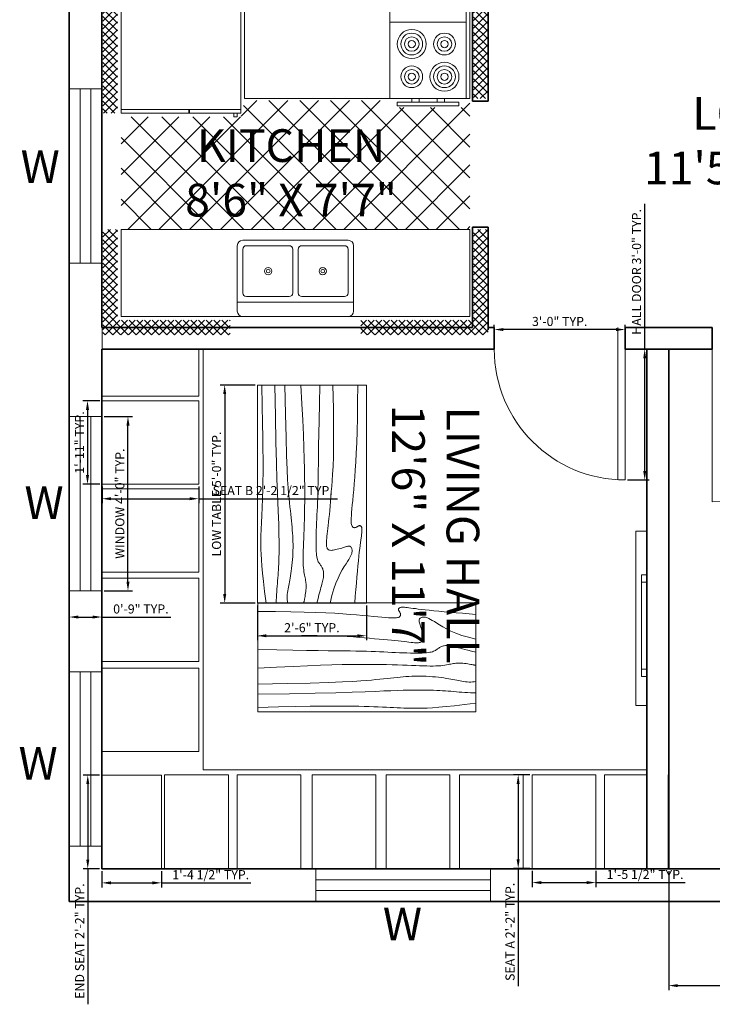
# Model space of a CAD drawing. Units: inches. Extents: x 1642 to 5612, y 1595 to 4064.
# Tile 4 of 6: x 2349 to 2539, y 1708 to 1979. Entities that reach past the tile are written whole.
import ezdxf

# ---------------------------------------------------------------- set-up
doc = ezdxf.new("R2010")
doc.units = ezdxf.units.IN
for name, color, linetype, lineweight in [('A-ANNO-DIMS', 2, 'Continuous', 18), ('A-ANNO-TEXT', 7, 'Continuous', 18), ('A-AREA-IDEN', 7, 'Continuous', 25), ('A-DOOR', 3, 'Continuous', 18), ('A-EQPM', 8, 'Continuous', 13), ('A-FLOR-FIXT', 9, 'Continuous', 18), ('A-FURN', 8, 'Continuous', 13), ('A-GLAZ', 4, 'Continuous', 18), ('A-WALL', 7, 'Continuous', 35)]:
    doc.layers.add(name, color=color, linetype=linetype, lineweight=lineweight)
doc.styles.get("Standard").update_dxf_attribs({"font": 'arial.ttf'})
doc.dimstyles.new('ISO-25', dxfattribs={"dimtxt": 2.5, "dimasz": 2.5, "dimexe": 1.25, "dimexo": 0.625, "dimtad": 1, "dimdec": 0, "dimlunit": 3, "dimtxsty": 'Standard', "dimcen": 2.5, "dimadec": 0, "dimazin": 0, "dimtfac": 1, "dimtdec": 0, "dimtmove": 0, "dimatfit": 3, "dimfxl": 1, "dimarcsym": 0})

# ---------------------------------------------------------------- blocks, each defined once
blk = doc.blocks.new('Kitchen Layout - 7 x 8 ft')
for p, q in [((-5, 81.32), (2.68, 89)), ((-5, 83.44), (0.56, 89)), ((-5, 85.56), (-1.56, 89)), ((-5, 87.68), (-3.68, 89)), ((-1, 84.97), (-5, 88.97)), ((-1, 82.85), (-5, 86.85)), ((1.09, 85), (-2.91, 89)), ((3.21, 85), (-0.79, 89)), ((0.81, 85), (4.81, 89)), ((5.34, 85), (1.34, 89)), ((2.93, 85), (6.93, 89)), ((7.46, 85), (3.46, 89)), ((5.05, 85), (9.05, 89)), ((9.58, 85), (5.58, 89)), ((7.17, 85), (11.17, 89)), ((11.7, 85), (7.7, 89)), ((9.29, 85), (13.29, 89)), ((13.82, 85), (9.82, 89)), ((11.41, 85), (15.41, 89)), ((15.94, 85), (11.94, 89)), ((13.53, 85), (17.53, 89)), ((18.06, 85), (14.06, 89)), ((15.65, 85), (19.65, 89)), ((20.18, 85), (16.18, 89)), ((17.78, 85), (21.78, 89)), ((22.31, 85), (18.31, 89)), ((19.9, 85), (23.9, 89)), ((24.43, 85), (20.43, 89)), ((22.02, 85), (26.02, 89)), ((26.55, 85), (22.55, 89)), ((24.14, 85), (28.14, 89)), ((28.67, 85), (24.67, 89)), ((26.26, 85), (30.26, 89)), ((30.79, 85), (26.79, 89)), ((28.38, 85), (32.38, 89)), ((32.91, 85), (28.91, 89)), ((30.5, 85), (34.5, 89)), ((35.03, 85), (31.03, 89)), ((32.63, 85), (36.63, 89)), ((37.16, 85), (33.16, 89)), ((34.75, 85), (38.75, 89)), ((39.28, 85), (35.28, 89)), ((36.87, 85), (40.87, 89)), ((41.4, 85), (37.4, 89)), ((38.99, 85), (42.99, 89)), ((43.52, 85), (39.52, 89)), ((41.11, 85), (45.11, 89)), ((45.64, 85), (41.64, 89)), ((43.23, 85), (47.23, 89)), ((47.76, 85), (43.76, 89)), ((45.35, 85), (49.35, 89)), ((49.88, 85), (45.88, 89)), ((47.47, 85), (51.47, 89)), ((52, 85), (48, 89)), ((49.6, 85), (53.6, 89)), ((54.13, 85), (50.13, 89)), ((51.72, 85), (55.72, 89)), ((56.25, 85), (52.25, 89)), ((53.84, 85), (57.84, 89)), ((58.37, 85), (54.37, 89)), ((55.96, 85), (59.96, 89)), ((60.49, 85), (56.49, 89)), ((58.08, 85), (62.08, 89)), ((62.61, 85), (58.61, 89)), ((60.2, 85), (64.2, 89)), ((64.73, 85), (60.73, 89)), ((62.32, 85), (66.32, 89)), ((66.85, 85), (62.85, 89)), ((64.45, 85), (68.45, 89)), ((68.97, 85), (64.97, 89)), ((66.57, 85), (70.57, 89)), ((71.1, 85), (67.1, 89)), ((68.69, 85), (72.69, 89)), ((73.22, 85), (69.22, 89)), ((70.81, 85), (74.81, 89)), ((75.34, 85), (71.34, 89)), ((72.93, 85), (76.93, 89)), ((77.46, 85), (73.46, 89)), ((75.05, 85), (79.05, 89)), ((79.58, 85), (75.58, 89)), ((77.17, 85), (81.17, 89)), ((81.7, 85), (77.7, 89)), ((79.29, 85), (83.29, 89)), ((83.82, 85), (79.82, 89)), ((81.42, 85), (85.42, 89)), ((85.95, 85), (81.95, 89)), ((83.54, 85), (87.54, 89)), ((88.07, 85), (84.07, 89)), ((85.66, 85), (89.66, 89)), ((90.19, 85), (86.19, 89)), ((87.78, 85), (91.78, 89)), ((92.31, 85), (88.31, 89)), ((89.9, 85), (93.9, 89)), ((94.43, 85), (90.43, 89)), ((92.02, 85), (96.02, 89)), ((96.55, 85), (92.55, 89)), ((94.14, 85), (98.14, 89)), ((101, 82.67), (94.67, 89)), ((96.27, 85), (100.27, 89)), ((101, 84.79), (96.79, 89)), ((97, 83.61), (101, 87.61)), ((101, 86.92), (98.92, 89)), ((-1, 80.73), (-5, 84.73)), ((34, 84), (96, 84)), ((34, 60), (34, 84)), ((96, 84), (96, 60)), ((97, 81.49), (101, 85.49)), ((101, 80.55), (97, 84.55)), ((-5, 79.19), (-1, 83.19)), ((-1, 78.61), (-5, 82.61)), ((97, 79.37), (101, 83.37)), ((101, 78.43), (97, 82.43)), ((-5, 77.07), (-1, 81.07)), ((-1, 76.49), (-5, 80.49)), ((-5, 74.95), (-1, 78.95)), ((74, 81), (95, 81)), ((97, 77.25), (101, 81.25)), ((101, 76.31), (97, 80.31)), ((97, 75.13), (101, 79.13)), ((-1, 74.36), (-5, 78.36)), ((-5, 72.83), (-1, 76.83)), ((-1, 72.24), (-5, 76.24)), ((101, 74.19), (97, 78.19)), ((97, 73.01), (101, 77.01)), ((101, 72.07), (97, 76.07)), ((-5, 70.71), (-1, 74.71)), ((-1, 70.12), (-5, 74.12)), ((97, 70.89), (101, 74.89)), ((101, 69.95), (97, 73.95)), ((-5, 68.59), (-1, 72.59)), ((-1, 68), (-5, 72)), ((-5, 66.47), (-1, 70.47)), ((97, 68.76), (101, 72.76)), ((101, 67.82), (97, 71.82)), ((97, 66.64), (101, 70.64)), ((-1, 65.88), (-5, 69.88)), ((-5, 64.35), (-1, 68.35)), ((-1, 63.76), (-5, 67.76)), ((101, 65.7), (97, 69.7)), ((97, 64.52), (101, 68.52)), ((-5, 62.22), (-1, 66.22)), ((-1, 61.64), (-5, 65.64)), ((101, 63.58), (97, 67.58)), ((97, 62.4), (101, 66.4)), ((101, 61.46), (97, 65.46)), ((-5, 60.1), (-1, 64.1)), ((-1, 59.52), (-5, 63.52)), ((97, 60.28), (101, 64.28)), ((100.34, 60), (97, 63.34)), ((-5, 57.98), (-1, 61.98)), ((-1, 57.39), (-5, 61.39)), ((-4.86, 56), (-1, 59.86)), ((96, 60), (34, 60)), ((80, 60), (80, 59)), ((82, 59), (82, 60)), ((87, 59), (87, 60)), ((89, 60), (89, 59)), ((98.22, 60), (97, 61.22)), ((98.84, 60), (101, 62.16)), ((100.96, 60), (101, 60.04)), ((-1.73, 56), (-5, 59.27)), ((-3.85, 56), (-5, 57.15)), ((-2.74, 56), (-1, 57.74)), ((0, 57), (33, 57)), ((10.4, 24), (45.9, 59.5)), ((18.88, 24), (54.38, 59.5)), ((27.37, 24), (62.87, 59.5)), ((33.03, 55.11), (37.41, 59.5)), ((67.71, 24), (33.68, 58.04)), ((35.85, 24), (71.35, 59.5)), ((76.2, 24), (40.7, 59.5)), ((44.34, 24), (77.84, 57.5)), ((84.68, 24), (49.18, 59.5)), ((52.82, 24), (86.32, 57.5)), ((93.17, 24), (57.67, 59.5)), ((61.31, 24), (96, 58.69)), ((96, 29.65), (66.15, 59.5)), ((96, 38.14), (76.64, 57.5)), ((96, 46.63), (85.13, 57.5)), ((96, 55.11), (93.57, 57.54)), ((0, 30.57), (24.43, 55)), ((0, 39.06), (15.94, 55)), ((0, 47.54), (7.46, 55)), ((1.91, 24), (32.91, 55)), ((33.77, 24), (2.77, 55)), ((42.26, 24), (11.26, 55)), ((50.74, 24), (19.74, 55)), ((59.23, 24), (28.23, 55)), ((31, 55), (31, 56)), ((32, 55), (31, 55)), ((32, 56), (32, 55)), ((25.29, 24), (0, 49.29)), ((69.79, 24), (96, 50.21)), ((16.8, 24), (0, 40.8)), ((78.28, 24), (96, 41.72)), ((86.76, 24), (96, 33.24)), ((8.32, 24), (0, 32.32)), ((95.25, 24), (96, 24.75)), ((-5, 21.92), (-2.92, 24)), ((-5, 19.8), (-1, 23.8)), ((-1, 19.21), (-5, 23.21)), ((-1, 21.33), (-3.67, 24)), ((-1, 23.45), (-1.55, 24)), ((0, 24), (96, 24)), ((0, 0), (0, 24)), ((96, 24), (96, 0)), ((97, 22.1), (98.9, 24)), ((97, 19.97), (101, 23.97)), ((101, 19.03), (97, 23.03)), ((97, 17.85), (101, 21.85)), ((101, 21.16), (98.16, 24)), ((101, 23.28), (100.28, 24)), ((-5, 17.68), (-1, 21.68)), ((-1, 17.09), (-5, 21.09)), ((-5, 15.55), (-1, 19.55)), ((-1, 14.97), (-5, 18.97)), ((101, 16.91), (97, 20.91)), ((97, 15.73), (101, 19.73)), ((-5, 13.43), (-1, 17.43)), ((-1, 12.85), (-5, 16.85)), ((47.25, 6.5), (47.25, 18.5)), ((48.75, 18.5), (48.75, 6.5)), ((101, 14.79), (97, 18.79)), ((97, 13.61), (101, 17.61)), ((101, 12.67), (97, 16.67)), ((-5, 11.31), (-1, 15.31)), ((-1, 10.73), (-5, 14.73)), ((97, 11.49), (101, 15.49)), ((101, 10.55), (97, 14.55)), ((-5, 9.19), (-1, 13.19)), ((-1, 8.6), (-5, 12.6)), ((-5, 7.07), (-1, 11.07)), ((97, 9.37), (101, 13.37)), ((101, 8.43), (97, 12.43)), ((97, 7.25), (101, 11.25)), ((-1, 6.48), (-5, 10.48)), ((-5, 4.95), (-1, 8.95)), ((-1, 4.36), (-5, 8.36)), ((101, 6.31), (97, 10.31)), ((97, 5.12), (101, 9.12)), ((101, 4.18), (97, 8.18)), ((-5, 2.83), (-1, 6.83)), ((-1, 2.24), (-5, 6.24)), ((97, 3), (101, 7)), ((101, 2.06), (97, 6.06)), ((-5, 0.71), (-1, 4.71)), ((-1, 0.12), (-5, 4.12)), ((64, 4), (32, 4)), ((93.24, -5), (101, 2.76)), ((97, 0.88), (101, 4.88)), ((101, -0.06), (97, 3.94)), ((-5, -1.42), (-1, 2.58)), ((2, -5), (-5, 2)), ((-5, -3.54), (-1, 0.46)), ((96, 0), (0, 0)), ((95.36, -5), (101, 0.64)), ((101, -2.18), (97, 1.82)), ((-0.12, -5), (-5, -0.12)), ((-2.25, -5), (-5, -2.25)), ((-4.34, -5), (-0.34, -1)), ((-2.22, -5), (1.78, -1)), ((-0.1, -5), (3.9, -1)), ((4.12, -5), (0.12, -1)), ((2.02, -5), (6.02, -1)), ((6.24, -5), (2.24, -1)), ((4.14, -5), (8.14, -1)), ((8.36, -5), (4.36, -1)), ((6.27, -5), (10.27, -1)), ((10.48, -5), (6.48, -1)), ((8.39, -5), (12.39, -1)), ((12.6, -5), (8.6, -1)), ((10.51, -5), (14.51, -1)), ((14.73, -5), (10.73, -1)), ((12.63, -5), (16.63, -1)), ((16.85, -5), (12.85, -1)), ((14.75, -5), (18.75, -1)), ((18.97, -5), (14.97, -1)), ((16.87, -5), (20.87, -1)), ((21.09, -5), (17.09, -1)), ((18.99, -5), (22.99, -1)), ((23.21, -5), (19.21, -1)), ((21.11, -5), (25.11, -1)), ((25.33, -5), (21.33, -1)), ((23.24, -5), (27.24, -1)), ((27.45, -5), (23.45, -1)), ((25.36, -5), (29.36, -1)), ((29.57, -5), (25.57, -1)), ((27.48, -5), (30, -2.48)), ((30, -3.3), (27.7, -1)), ((30, -1.18), (29.82, -1)), ((66, -2.54), (67.54, -1)), ((66, -4.66), (69.66, -1)), ((69.88, -5), (66, -1.12)), ((67.78, -5), (71.78, -1)), ((72, -5), (68, -1)), ((69.9, -5), (73.9, -1)), ((74.12, -5), (70.12, -1)), ((72.03, -5), (76.03, -1)), ((76.24, -5), (72.24, -1)), ((74.15, -5), (78.15, -1)), ((78.36, -5), (74.36, -1)), ((76.27, -5), (80.27, -1)), ((80.49, -5), (76.49, -1)), ((78.39, -5), (82.39, -1)), ((82.61, -5), (78.61, -1)), ((80.51, -5), (84.51, -1)), ((84.73, -5), (80.73, -1)), ((82.63, -5), (86.63, -1)), ((86.85, -5), (82.85, -1)), ((84.75, -5), (88.75, -1)), ((88.97, -5), (84.97, -1)), ((86.88, -5), (90.88, -1)), ((91.09, -5), (87.09, -1)), ((89, -5), (93, -1)), ((93.21, -5), (89.21, -1)), ((91.12, -5), (95.12, -1)), ((95.34, -5), (91.34, -1)), ((97.46, -5), (93.46, -1)), ((99.58, -5), (95.58, -1)), ((101, -4.3), (97, -0.3)), ((97.48, -5), (101, -1.48)), ((-4.37, -5), (-5, -4.37)), ((29.6, -5), (30, -4.6)), ((67.76, -5), (66, -3.24)), ((99.6, -5), (101, -3.6))]:
    blk.add_line(p, q)
for points in [[(0, 56), (0, 84), (33, 84), (33, 56)], [(74, 60), (74, 84), (95, 84), (95, 60)], [(76, 58), (76, 59), (93, 59), (93, 58)]]:
    blk.add_lwpolyline(points, close=True)
for points in [[(32, 1.5), (32, 19.5)], [(33.5, 21), (62.5, 21)], [(34.5, 19.5), (46.25, 19.5)], [(49.75, 19.5), (61.5, 19.5)], [(64, 19.5), (64, 1.5)], [(33.5, 6.5), (33.5, 18.5)], [(62.5, 18.5), (62.5, 6.5)], [(46.25, 5.5), (34.5, 5.5)], [(61.5, 5.5), (49.75, 5.5)], [(62.5, 0), (33.5, 0)]]:
    blk.add_lwpolyline(points)
for centre, radius in [((80, 75), 4), ((80, 75), 3), ((80, 75), 2), ((80, 75), 1), ((89, 75), 3), ((89, 75), 2), ((89, 75), 1), ((80, 66), 3), ((80, 66), 2), ((89, 66), 4), ((89, 66), 3), ((89, 66), 2), ((80, 66), 1), ((89, 66), 1), ((40.5, 12.5), 1), ((40.5, 12.5), 0.5), ((55.5, 12.5), 1), ((55.5, 12.5), 0.5)]:
    blk.add_circle(centre, radius)
for centre, radius, start, end in [((33.5, 19.5), 1.5, 90, 180), ((34.5, 18.5), 1, 90, 180), ((46.25, 18.5), 1, 0, 90), ((49.75, 18.5), 1, 90, 180), ((61.5, 18.5), 1, 0, 90), ((62.5, 19.5), 1.5, 0, 90), ((34.5, 6.5), 1, 180, 270), ((46.25, 6.5), 1, 270, 0), ((49.75, 6.5), 1, 180, 270), ((61.5, 6.5), 1, 270, 0), ((33.5, 1.5), 1.5, 180, 270), ((62.5, 1.5), 1.5, 270, 0)]:
    blk.add_arc(centre, radius, start, end)
blk = doc.blocks.new('Table - Rectangular Woodgrain 60 x 30 in.')
for p, q in [((0, 0), (0, -30)), ((60, 0), (0, 0)), ((60, -30), (60, 0)), ((0, -30), (60, -30))]:
    blk.add_line(p, q)
for points in [[(0, -2.4), (4.8155, -2.418), (9.0302, -2.4688), (12.709, -2.5477), (15.9167, -2.65), (18.7181, -2.7711), (21.1781, -2.9063), (23.3616, -3.0508), (25.3333, -3.2), (27.1477, -3.3495), (28.8172, -3.4958), (30.3437, -3.636), (31.7291, -3.7667), (32.9756, -3.8849), (34.0849, -3.9875), (35.059, -4.0714), (35.9, -4.1334), (36.6114, -4.1711), (37.2041, -4.1854), (37.6906, -4.1779), (38.0833, -4.15), (38.3948, -4.1034), (38.6375, -4.0396), (38.8239, -3.9602), (38.9666, -3.8667), (39.0764, -3.7608), (39.1573, -3.6448), (39.2116, -3.521), (39.2416, -3.3917), (39.2498, -3.2593), (39.2385, -3.1261), (39.21, -2.9944), (39.1666, -2.8667), (39.111, -2.7447), (39.0468, -2.6281), (38.978, -2.5163), (38.9083, -2.4083), (38.8418, -2.3035), (38.7823, -2.201), (38.7337, -2.1001), (38.7, -2), (38.6844, -1.9003), (38.6875, -1.8021), (38.7094, -1.707), (38.75, -1.6167), (38.8094, -1.5326), (38.8875, -1.4563), (38.9844, -1.3893), (39.1, -1.3333), (39.2351, -1.2896), (39.3937, -1.2583), (39.5804, -1.2396), (39.8, -1.2333), (40.057, -1.2396), (40.3562, -1.2583), (40.7023, -1.2896), (41.1, -1.3333), (41.5547, -1.3895), (42.0755, -1.4573), (42.6721, -1.5361), (43.3542, -1.625), (44.1316, -1.7233), (45.014, -1.8302), (46.0114, -1.9449), (47.1333, -2.0667), (48.3862, -2.1947), (49.7625, -2.3281), (51.2513, -2.4663), (52.8416, -2.6083), (54.5226, -2.7535), (56.2833, -2.9011), (58.1127, -3.0501), (60, -3.2)], [(0, -9.2), (6.5759, -9.0858), (11.9385, -9.0365), (16.2527, -9.0418), (19.6833, -9.0917), (22.3952, -9.1759), (24.5531, -9.2844), (26.322, -9.4069), (27.8666, -9.5333), (29.3241, -9.6553), (30.7203, -9.7719), (32.0532, -9.8837), (33.3208, -9.9917), (34.5213, -10.0965), (35.6526, -10.199), (36.7128, -10.2999), (37.7, -10.4), (38.6129, -10.4996), (39.4531, -10.5969), (40.223, -10.6895), (40.925, -10.775), (41.5613, -10.8512), (42.1344, -10.9156), (42.6465, -10.966), (43.1, -11), (43.4976, -11.0158), (43.8437, -11.0136), (44.143, -10.9942), (44.4, -10.9583), (44.6195, -10.9069), (44.8062, -10.8406), (44.9648, -10.7603), (45.1, -10.6667), (45.2155, -10.5598), (45.3114, -10.4365), (45.3871, -10.2929), (45.4416, -10.125), (45.4743, -9.929), (45.4844, -9.7011), (45.4709, -9.4371), (45.4333, -9.1333), (45.3716, -8.7883), (45.2896, -8.4104), (45.1919, -8.0107), (45.0833, -7.6), (44.9685, -7.1893), (44.8521, -6.7896), (44.7388, -6.4117), (44.6333, -6.0667), (44.54, -5.7628), (44.4614, -5.4979), (44.4001, -5.2675), (44.3583, -5.0667), (44.3384, -4.8909), (44.3427, -4.7354), (44.3736, -4.5956), (44.4333, -4.4667), (44.5236, -4.3453), (44.6427, -4.2333), (44.7884, -4.1339), (44.9583, -4.05), (45.1501, -3.9849), (45.3614, -3.9417), (45.59, -3.9234), (45.8333, -3.9333), (46.0915, -3.9749), (46.3734, -4.0531), (46.6906, -4.1736), (47.0542, -4.3417), (47.4756, -4.5629), (47.9661, -4.8427), (48.5372, -5.1866), (49.2, -5.6), (49.9676, -6.0844), (50.8594, -6.625), (51.8965, -7.2031), (53.1, -7.8), (54.491, -8.3969), (56.0906, -8.975), (57.9199, -9.5156), (60, -10)], [(0, -12.8), (5.1847, -12.9322), (9.6213, -13.0323), (13.3963, -13.1059), (16.5958, -13.1583), (19.3063, -13.1952), (21.614, -13.2219), (23.6054, -13.2439), (25.3666, -13.2667), (26.9728, -13.2947), (28.4531, -13.3281), (29.8256, -13.3663), (31.1083, -13.4083), (32.3191, -13.4535), (33.476, -13.501), (34.597, -13.5501), (35.7, -13.6), (36.7984, -13.6497), (37.8875, -13.6979), (38.9578, -13.743), (40, -13.7833), (41.0047, -13.8174), (41.9625, -13.8438), (42.864, -13.8607), (43.7, -13.8667), (44.4631, -13.8604), (45.1552, -13.8417), (45.7801, -13.8104), (46.3416, -13.7667), (46.8439, -13.7104), (47.2906, -13.6417), (47.6858, -13.5604), (48.0333, -13.4667), (48.3375, -13.3608), (48.6042, -13.2448), (48.8396, -13.121), (49.05, -12.9917), (49.2417, -12.8593), (49.4208, -12.7261), (49.5937, -12.5944), (49.7667, -12.4667), (49.9452, -12.3451), (50.1323, -12.2313), (50.3303, -12.1268), (50.5416, -12.0333), (50.7686, -11.9524), (51.0135, -11.8854), (51.2788, -11.8341), (51.5666, -11.8), (51.8785, -11.7843), (52.2116, -11.7865), (52.562, -11.8059), (52.926, -11.8417), (53.2998, -11.8931), (53.6795, -11.9594), (54.0614, -12.0397), (54.4416, -12.1333), (54.8223, -12.2401), (55.2293, -12.3625), (55.6942, -12.5037), (56.2489, -12.6667), (56.9251, -12.8547), (57.7545, -13.0708), (58.7689, -13.3182), (60, -13.6)], [(0, -18), (5.124, -17.7273), (9.6609, -17.5057), (13.6705, -17.3303), (17.2125, -17.1958), (20.3467, -17.0973), (23.1328, -17.0297), (25.6307, -16.9878), (27.9, -16.9667), (29.9928, -16.9617), (31.9302, -16.9703), (33.7254, -16.9907), (35.3917, -17.0208), (36.9423, -17.0588), (38.3906, -17.1026), (39.7499, -17.1503), (41.0333, -17.2), (42.2519, -17.2496), (43.4073, -17.2969), (44.4986, -17.3395), (45.525, -17.375), (46.4858, -17.4012), (47.3802, -17.4156), (48.2074, -17.416), (48.9667, -17.4), (49.6583, -17.3662), (50.2872, -17.3167), (50.8595, -17.2547), (51.3812, -17.1833), (51.8584, -17.1057), (52.2971, -17.025), (52.7034, -16.9443), (53.0833, -16.8667), (53.443, -16.7951), (53.789, -16.7313), (54.128, -16.6768), (54.4666, -16.6334), (54.8115, -16.6024), (55.1693, -16.5854), (55.5465, -16.5841), (55.95, -16.6), (56.3828, -16.6337), (56.8346, -16.6823), (57.2915, -16.7418), (57.7396, -16.8084), (58.165, -16.878), (58.5539, -16.9469), (58.8924, -17.0111), (59.1666, -17.0667), (59.3679, -17.1107), (59.5078, -17.1438), (59.6032, -17.1675), (59.6708, -17.1833), (59.7275, -17.193), (59.7901, -17.1979), (59.8753, -17.1998), (60, -17.2)], [(0, -22.4), (8.0098, -22.2501), (14.4094, -22.1011), (19.4168, -21.9535), (23.25, -21.8083), (26.1269, -21.6663), (28.2656, -21.5281), (29.884, -21.3947), (31.2, -21.2667), (32.3967, -21.1448), (33.5172, -21.0292), (34.5697, -20.9198), (35.5625, -20.8167), (36.5037, -20.7198), (37.4015, -20.6292), (38.2642, -20.5448), (39.1, -20.4667), (39.9164, -20.3951), (40.7187, -20.3313), (41.5117, -20.2768), (42.3, -20.2333), (43.0883, -20.2024), (43.8812, -20.1854), (44.6836, -20.1841), (45.5, -20.2), (46.3328, -20.234), (47.1747, -20.2844), (48.0163, -20.3488), (48.8479, -20.425), (49.66, -20.5106), (50.4429, -20.6031), (51.1872, -20.7004), (51.8833, -20.8), (52.5246, -20.8999), (53.1166, -20.9995), (53.6681, -21.0983), (54.1875, -21.1958), (54.6834, -21.2919), (55.1646, -21.3859), (55.6394, -21.4777), (56.1167, -21.5667), (56.6028, -21.6515), (57.0961, -21.7266), (57.5929, -21.7852), (58.0896, -21.8208), (58.5823, -21.8268), (59.0674, -21.7964), (59.5412, -21.723), (60, -21.6)], [(0, -25.2), (8.6355, -25.0504), (15.7026, -24.9031), (21.4049, -24.7606), (25.9458, -24.625), (29.529, -24.4988), (32.3578, -24.3844), (34.6359, -24.284), (36.5667, -24.2), (38.3213, -24.1341), (39.9417, -24.0854), (41.437, -24.0523), (42.8167, -24.0333), (44.0901, -24.0268), (45.2667, -24.0313), (46.3557, -24.0451), (47.3667, -24.0667), (48.309, -24.0947), (49.1928, -24.1287), (50.0284, -24.168), (50.826, -24.2125), (51.5959, -24.2617), (52.3483, -24.3151), (53.0935, -24.3725), (53.8417, -24.4334), (54.6009, -24.497), (55.3699, -24.561), (56.1454, -24.6226), (56.9239, -24.6792), (57.7021, -24.7279), (58.4764, -24.7662), (59.2435, -24.7911), (60, -24.8)], [(0, -28.8), (5.6867, -28.6681), (10.45, -28.5698), (14.407, -28.5012), (17.675, -28.4584), (20.3711, -28.4374), (22.6125, -28.4344), (24.5164, -28.4455), (26.2, -28.4667), (27.762, -28.4947), (29.2276, -28.5281), (30.6033, -28.5663), (31.8958, -28.6084), (33.1118, -28.6535), (34.2578, -28.7011), (35.3405, -28.7501), (36.3666, -28.8), (37.3443, -28.8497), (38.288, -28.8974), (39.2137, -28.9412), (40.1375, -28.9792), (41.0753, -29.0093), (42.0432, -29.0297), (43.0572, -29.0384), (44.1333, -29.0333), (45.2936, -29.0114), (46.5843, -28.9641), (48.0579, -28.8816), (49.7666, -28.7542), (51.7629, -28.5721), (54.0989, -28.3255), (56.8272, -28.0048), (60, -27.6)]]:
    blk.add_lwpolyline(points)
blk = doc.blocks.new('WIN-48x9')
for p, q in [((0, 48), (0, 0)), ((9, 48), (0, 48)), ((3, 48), (3, 0)), ((6, 0), (6, 48)), ((9, 0), (9, 48)), ((0, 0), (9, 0))]:
    blk.add_line(p, q)
blk = doc.blocks.new('DOOR-SWING-36')
for p, q in [((36, 2), (0, 2)), ((36, 0), (0, 0))]:
    blk.add_line(p, q)
blk.add_arc((36, 0), 36, 90, 180)
blk = doc.blocks.new('SEATING-CUSHION-NARROW')
blk.add_lwpolyline([(0, 17.53), (25.79, 17.53), (25.79, 0), (0, 0)], close=True)
blk = doc.blocks.new('SEATING-CUSHION-WIDE')
blk.add_lwpolyline([(0, 26.61), (22.95, 26.61), (22.95, 0), (0, 0)], close=True)
blk = doc.blocks.new('SEATING-CUSHION-END')
blk.add_line((0, 0), (25.79, 0))
blk.add_lwpolyline([(0, 0), (0, 16.43), (25.79, 16.43), (25.79, 0)])
blk = doc.blocks.new('*D28')
at = {"layer": 'A-ANNO-DIMS', "color": 0, "lineweight": -2, "transparency": 16777216}
for p, q in [((2413.45, 1878.76), (2403.83, 1878.76)), ((2405.08, 1876.26), (2405.08, 1821.26)), ((2413.45, 1818.76), (2403.83, 1818.76))]:
    blk.add_line(p, q, dxfattribs=at)
at = {"layer": 'A-ANNO-DIMS', "color": 0, "transparency": 16777216}
for points in [[(2404.66, 1876.26), (2405.5, 1876.26), (2405.08, 1878.76)], [(2404.66, 1821.26), (2405.5, 1821.26), (2405.08, 1818.76)]]:
    blk.add_solid(points, dxfattribs=at)
at = {"layer": 'Defpoints', "color": 0, "transparency": 16777216}
for p in [(2414.08, 1878.76), (2405.08, 1818.76), (2414.08, 1818.76)]:
    blk.add_point(p, dxfattribs=at)
at = {"layer": 'A-ANNO-DIMS', "color": 0, "transparency": 16777216, "insert": (2403.16, 1848.76), "char_height": 2.5, "attachment_point": 5, "rotation": 90}
blk.add_mtext('LOW TABLE 5\'-0" TYP.', dxfattribs=at)
blk = doc.blocks.new('*D29')
at = {"layer": 'A-ANNO-DIMS', "color": 0, "lineweight": -2, "transparency": 16777216}
for p, q in [((2414.08, 1818.14), (2414.08, 1808.51)), ((2444.08, 1818.14), (2444.08, 1808.51)), ((2416.58, 1809.76), (2441.58, 1809.76))]:
    blk.add_line(p, q, dxfattribs=at)
at = {"layer": 'A-ANNO-DIMS', "color": 0, "transparency": 16777216}
for points in [[(2416.58, 1810.18), (2416.58, 1809.34), (2414.08, 1809.76)], [(2441.58, 1810.18), (2441.58, 1809.34), (2444.08, 1809.76)]]:
    blk.add_solid(points, dxfattribs=at)
at = {"layer": 'Defpoints', "color": 0, "transparency": 16777216}
for p in [(2414.08, 1818.76), (2444.08, 1818.76), (2444.08, 1809.76)]:
    blk.add_point(p, dxfattribs=at)
at = {"layer": 'A-ANNO-DIMS', "color": 0, "transparency": 16777216, "insert": (2429.08, 1811.66), "char_height": 2.5, "attachment_point": 5}
blk.add_mtext('2\'-6" TYP.', dxfattribs=at)
blk = doc.blocks.new('*D30')
at = {"layer": 'A-ANNO-DIMS', "color": 0, "lineweight": -2, "transparency": 16777216}
for p, q in [((2371.9, 1870.12), (2379.72, 1870.12)), ((2378.47, 1824.62), (2378.47, 1867.62)), ((2371.9, 1822.12), (2379.72, 1822.12))]:
    blk.add_line(p, q, dxfattribs=at)
at = {"layer": 'A-ANNO-DIMS', "color": 0, "transparency": 16777216}
for points in [[(2378.06, 1867.62), (2378.89, 1867.62), (2378.47, 1870.12)], [(2378.06, 1824.62), (2378.89, 1824.62), (2378.47, 1822.12)]]:
    blk.add_solid(points, dxfattribs=at)
at = {"layer": 'Defpoints', "color": 0, "transparency": 16777216}
for p in [(2371.27, 1870.12), (2378.47, 1870.12), (2371.27, 1822.12)]:
    blk.add_point(p, dxfattribs=at)
at = {"layer": 'A-ANNO-DIMS', "color": 0, "transparency": 16777216, "insert": (2376.55, 1846.12), "char_height": 2.5, "attachment_point": 5, "rotation": 90}
blk.add_mtext('WINDOW 4\'-0" TYP.', dxfattribs=at)
blk = doc.blocks.new('*D31')
at = {"layer": 'A-ANNO-DIMS', "color": 0, "lineweight": -2, "transparency": 16777216}
for p, q in [((2362.27, 1821.49), (2362.27, 1813.67)), ((2371.27, 1821.49), (2371.27, 1813.67)), ((2364.77, 1814.92), (2368.77, 1814.92)), ((2371.27, 1814.92), (2390.26, 1814.92))]:
    blk.add_line(p, q, dxfattribs=at)
at = {"layer": 'A-ANNO-DIMS', "color": 0, "transparency": 16777216}
for points in [[(2364.77, 1815.33), (2364.77, 1814.5), (2362.27, 1814.92)], [(2368.77, 1815.33), (2368.77, 1814.5), (2371.27, 1814.92)]]:
    blk.add_solid(points, dxfattribs=at)
at = {"layer": 'Defpoints', "color": 0, "transparency": 16777216}
for p in [(2362.27, 1822.12), (2371.27, 1822.12), (2371.27, 1814.92)]:
    blk.add_point(p, dxfattribs=at)
at = {"layer": 'A-ANNO-DIMS', "color": 0, "transparency": 16777216, "insert": (2382.02, 1816.82), "char_height": 2.5, "attachment_point": 5}
blk.add_mtext('0\'-9" TYP.', dxfattribs=at)
blk = doc.blocks.new('*D34')
at = {"layer": 'A-ANNO-DIMS', "color": 0, "lineweight": -2, "transparency": 16777216}
for p, q in [((2489.09, 1771.5), (2484.6, 1771.5)), ((2485.85, 1769), (2485.85, 1748.21)), ((2489.09, 1745.71), (2484.6, 1745.71)), ((2485.85, 1745.71), (2485.85, 1713.34))]:
    blk.add_line(p, q, dxfattribs=at)
at = {"layer": 'A-ANNO-DIMS', "color": 0, "transparency": 16777216}
for points in [[(2485.43, 1769), (2486.26, 1769), (2485.85, 1771.5)], [(2485.43, 1748.21), (2486.26, 1748.21), (2485.85, 1745.71)]]:
    blk.add_solid(points, dxfattribs=at)
at = {"layer": 'Defpoints', "color": 0, "transparency": 16777216}
for p in [(2489.71, 1771.5), (2485.85, 1745.71), (2489.71, 1745.71)]:
    blk.add_point(p, dxfattribs=at)
at = {"layer": 'A-ANNO-DIMS', "color": 0, "transparency": 16777216, "insert": (2483.93, 1728.28), "char_height": 2.5, "attachment_point": 5, "rotation": 90}
blk.add_mtext('SEAT A 2\'-2" TYP.', dxfattribs=at)
blk = doc.blocks.new('*D35')
at = {"layer": 'A-ANNO-DIMS', "color": 0, "lineweight": -2, "transparency": 16777216}
for p, q in [((2489.71, 1745.09), (2489.71, 1740.59)), ((2507.24, 1745.09), (2507.24, 1740.59)), ((2492.21, 1741.84), (2504.74, 1741.84)), ((2507.24, 1741.84), (2531.82, 1741.84))]:
    blk.add_line(p, q, dxfattribs=at)
at = {"layer": 'A-ANNO-DIMS', "color": 0, "transparency": 16777216}
for points in [[(2492.21, 1742.26), (2492.21, 1741.43), (2489.71, 1741.84)], [(2504.74, 1742.26), (2504.74, 1741.43), (2507.24, 1741.84)]]:
    blk.add_solid(points, dxfattribs=at)
at = {"layer": 'Defpoints', "color": 0, "transparency": 16777216}
for p in [(2489.71, 1745.71), (2507.24, 1745.71), (2507.24, 1741.84)]:
    blk.add_point(p, dxfattribs=at)
at = {"layer": 'A-ANNO-DIMS', "color": 0, "transparency": 16777216, "insert": (2520.78, 1743.76), "char_height": 2.5, "attachment_point": 5}
blk.add_mtext('1\'-5 1/2" TYP.', dxfattribs=at)
blk = doc.blocks.new('*D36')
at = {"layer": 'A-ANNO-DIMS', "color": 0, "lineweight": -2, "transparency": 16777216}
for p, q in [((2371.32, 1850.85), (2371.32, 1846.23)), ((2397.93, 1850.85), (2397.93, 1846.23)), ((2373.82, 1847.48), (2395.43, 1847.48)), ((2397.93, 1847.48), (2436.13, 1847.48))]:
    blk.add_line(p, q, dxfattribs=at)
at = {"layer": 'A-ANNO-DIMS', "color": 0, "transparency": 16777216}
for points in [[(2373.82, 1847.9), (2373.82, 1847.07), (2371.32, 1847.48)], [(2395.43, 1847.9), (2395.43, 1847.07), (2397.93, 1847.48)]]:
    blk.add_solid(points, dxfattribs=at)
at = {"layer": 'Defpoints', "color": 0, "transparency": 16777216}
for p in [(2371.32, 1851.47), (2397.93, 1851.47), (2397.93, 1847.48)]:
    blk.add_point(p, dxfattribs=at)
at = {"layer": 'A-ANNO-DIMS', "color": 0, "transparency": 16777216, "insert": (2418.28, 1849.4), "char_height": 2.5, "attachment_point": 5}
blk.add_mtext('SEAT B 2\'-2 1/2" TYP.', dxfattribs=at)
blk = doc.blocks.new('*D37')
at = {"layer": 'A-ANNO-DIMS', "color": 0, "lineweight": -2, "transparency": 16777216}
for p, q in [((2370.7, 1874.42), (2366.08, 1874.42)), ((2367.33, 1871.92), (2367.33, 1853.97)), ((2370.7, 1851.47), (2366.08, 1851.47))]:
    blk.add_line(p, q, dxfattribs=at)
at = {"layer": 'A-ANNO-DIMS', "color": 0, "transparency": 16777216}
for points in [[(2366.91, 1871.92), (2367.75, 1871.92), (2367.33, 1874.42)], [(2366.91, 1853.97), (2367.75, 1853.97), (2367.33, 1851.47)]]:
    blk.add_solid(points, dxfattribs=at)
at = {"layer": 'Defpoints', "color": 0, "transparency": 16777216}
for p in [(2371.32, 1874.42), (2367.33, 1851.47), (2371.32, 1851.47)]:
    blk.add_point(p, dxfattribs=at)
at = {"layer": 'A-ANNO-DIMS', "color": 0, "transparency": 16777216, "insert": (2365.45, 1862.95), "char_height": 2.5, "attachment_point": 5, "rotation": 90}
blk.add_mtext('1\'-11" TYP.', dxfattribs=at)
blk = doc.blocks.new('*D38')
at = {"layer": 'A-ANNO-DIMS', "color": 0, "lineweight": -2, "transparency": 16777216}
for p, q in [((2370.65, 1771.43), (2366.15, 1771.43)), ((2367.4, 1768.93), (2367.4, 1748.14)), ((2370.65, 1745.64), (2366.15, 1745.64)), ((2367.4, 1745.64), (2367.4, 1708.34))]:
    blk.add_line(p, q, dxfattribs=at)
at = {"layer": 'A-ANNO-DIMS', "color": 0, "transparency": 16777216}
for points in [[(2366.99, 1768.93), (2367.82, 1768.93), (2367.4, 1771.43)], [(2366.99, 1748.14), (2367.82, 1748.14), (2367.4, 1745.64)]]:
    blk.add_solid(points, dxfattribs=at)
at = {"layer": 'Defpoints', "color": 0, "transparency": 16777216}
for p in [(2371.27, 1771.43), (2367.4, 1745.64), (2371.27, 1745.64)]:
    blk.add_point(p, dxfattribs=at)
at = {"layer": 'A-ANNO-DIMS', "color": 0, "transparency": 16777216, "insert": (2365.49, 1725.74), "char_height": 2.5, "attachment_point": 5, "rotation": 90}
blk.add_mtext('END SEAT 2\'-2" TYP.', dxfattribs=at)
blk = doc.blocks.new('*D39')
at = {"layer": 'A-ANNO-DIMS', "color": 0, "lineweight": -2, "transparency": 16777216}
for p, q in [((2371.27, 1745.01), (2371.27, 1740.52)), ((2387.7, 1745.01), (2387.7, 1740.52)), ((2373.77, 1741.77), (2385.2, 1741.77)), ((2387.7, 1741.77), (2412.28, 1741.77))]:
    blk.add_line(p, q, dxfattribs=at)
at = {"layer": 'A-ANNO-DIMS', "color": 0, "transparency": 16777216}
for points in [[(2373.77, 1742.18), (2373.77, 1741.35), (2371.27, 1741.77)], [(2385.2, 1742.18), (2385.2, 1741.35), (2387.7, 1741.77)]]:
    blk.add_solid(points, dxfattribs=at)
at = {"layer": 'Defpoints', "color": 0, "transparency": 16777216}
for p in [(2371.27, 1745.64), (2387.7, 1745.64), (2387.7, 1741.77)]:
    blk.add_point(p, dxfattribs=at)
at = {"layer": 'A-ANNO-DIMS', "color": 0, "transparency": 16777216, "insert": (2401.24, 1743.69), "char_height": 2.5, "attachment_point": 5}
blk.add_mtext('1\'-4 1/2" TYP.', dxfattribs=at)
blk = doc.blocks.new('*D48')
at = {"layer": 'A-ANNO-DIMS', "color": 0, "lineweight": -2, "transparency": 16777216}
for p, q in [((2520.67, 1888.64), (2520.67, 1928.64)), ((2515.9, 1888.64), (2521.92, 1888.64)), ((2520.67, 1855.14), (2520.67, 1886.14)), ((2515.9, 1852.64), (2521.92, 1852.64))]:
    blk.add_line(p, q, dxfattribs=at)
at = {"layer": 'A-ANNO-DIMS', "color": 0, "transparency": 16777216}
for points in [[(2520.26, 1886.14), (2521.09, 1886.14), (2520.67, 1888.64)], [(2520.26, 1855.14), (2521.09, 1855.14), (2520.67, 1852.64)]]:
    blk.add_solid(points, dxfattribs=at)
at = {"layer": 'Defpoints', "color": 0, "transparency": 16777216}
for p in [(2515.27, 1888.64), (2520.67, 1888.64), (2515.27, 1852.64)]:
    blk.add_point(p, dxfattribs=at)
at = {"layer": 'A-ANNO-DIMS', "color": 0, "transparency": 16777216, "insert": (2518.75, 1909.89), "char_height": 2.5, "attachment_point": 5, "rotation": 90}
blk.add_mtext('HALL DOOR 3\'-0" TYP.', dxfattribs=at)
blk = doc.blocks.new('*D49')
at = {"layer": 'A-ANNO-DIMS', "color": 0, "lineweight": -2, "transparency": 16777216}
for p, q in [((2479.27, 1889.26), (2479.27, 1895.29)), ((2515.27, 1889.26), (2515.27, 1895.29)), ((2512.77, 1894.04), (2481.77, 1894.04))]:
    blk.add_line(p, q, dxfattribs=at)
at = {"layer": 'A-ANNO-DIMS', "color": 0, "transparency": 16777216}
for points in [[(2481.77, 1894.45), (2481.77, 1893.62), (2479.27, 1894.04)], [(2512.77, 1894.45), (2512.77, 1893.62), (2515.27, 1894.04)]]:
    blk.add_solid(points, dxfattribs=at)
at = {"layer": 'Defpoints', "color": 0, "transparency": 16777216}
for p in [(2479.27, 1894.04), (2479.27, 1888.64), (2515.27, 1888.64)]:
    blk.add_point(p, dxfattribs=at)
at = {"layer": 'A-ANNO-DIMS', "color": 0, "transparency": 16777216, "insert": (2497.27, 1895.94), "char_height": 2.5, "attachment_point": 5}
blk.add_mtext('3\'-0" TYP.', dxfattribs=at)
blk = doc.blocks.new('*D56')
at = {"layer": 'A-ANNO-DIMS', "color": 0, "lineweight": -2, "transparency": 16777216}
for p, q in [((2527.27, 1745.01), (2527.27, 1712.24)), ((2648.27, 1745.01), (2648.27, 1712.24)), ((2529.77, 1713.49), (2645.77, 1713.49))]:
    blk.add_line(p, q, dxfattribs=at)
at = {"layer": 'A-ANNO-DIMS', "color": 0, "transparency": 16777216}
for points in [[(2529.77, 1713.9), (2529.77, 1713.07), (2527.27, 1713.49)], [(2645.77, 1713.9), (2645.77, 1713.07), (2648.27, 1713.49)]]:
    blk.add_solid(points, dxfattribs=at)
at = {"layer": 'Defpoints', "color": 0, "transparency": 16777216}
for p in [(2527.27, 1745.64), (2648.27, 1745.64), (2648.27, 1713.49)]:
    blk.add_point(p, dxfattribs=at)
at = {"layer": 'A-ANNO-DIMS', "color": 0, "transparency": 16777216, "insert": (2587.77, 1715.39), "char_height": 2.5, "attachment_point": 5}
blk.add_mtext('10\'-1"', dxfattribs=at)

msp = doc.modelspace()

# ---------------------------------------------------------------- linework, layer by layer
at = {"layer": 'A-DOOR'}
for p, q in [((2513.27, 1888.64), (2513.27, 1894.64)), ((2539.27, 1888.64), (2539.27, 1846.64))]:
    msp.add_line(p, q, dxfattribs=at)
msp.add_arc((2539.27, 1888.64), 42, 270, 360, dxfattribs=at)
at = {"layer": 'A-EQPM'}
for p, q in [((2518.19, 1790.56), (2518.19, 1838.56)), ((2521.19, 1838.56), (2518.19, 1838.56)), ((2521.19, 1838.56), (2521.19, 1826.56)), ((2521.19, 1826.56), (2519.81, 1826.56)), ((2519.81, 1826.56), (2519.81, 1824.56)), ((2519.81, 1826.56), (2519.81, 1798.56)), ((2519.81, 1824.56), (2521.27, 1824.56)), ((2521.27, 1824.56), (2521.27, 1800.56)), ((2521.27, 1800.56), (2519.81, 1800.56)), ((2519.81, 1798.56), (2521.27, 1798.56)), ((2518.19, 1790.56), (2521.19, 1790.56))]:
    msp.add_line(p, q, dxfattribs=at)
at = {"layer": 'A-FURN'}
for p in [(2399.17, 1888.64), (2521.27, 1772.9)]:
    msp.add_line(p, (2399.17, 1772.9), dxfattribs=at)
for points in [[(2397.93, 1888.64), (2397.93, 1875.68), (2371.32, 1875.68), (2371.32, 1898.63)], [(2527.14, 1771.5), (2527.14, 1745.71), (2509.61, 1745.71), (2509.61, 1771.5), (2521.27, 1771.5)]]:
    msp.add_lwpolyline(points, dxfattribs=at)
at = {"layer": 'A-GLAZ'}
for p, q in [((2521.27, 1829.69), (2521.27, 1781.69)), ((2527.27, 1781.69), (2527.27, 1829.69))]:
    msp.add_line(p, q, dxfattribs=at)
at = {"layer": 'A-WALL'}
for p, q in [((2362.27, 2120.64), (2362.27, 1736.64)), ((2371.27, 1985.64), (2371.27, 1894.64)), ((2473.27, 1985.64), (2473.27, 1956.89)), ((2477.56, 1985.23), (2477.56, 1956.89)), ((2473.27, 1956.89), (2477.56, 1956.89)), ((2395.27, 1954.61), (2395.27, 1953.61)), ((2477.56, 1922.21), (2473.27, 1922.21)), ((2473.27, 1922.21), (2473.27, 1894.64)), ((2477.56, 1922.21), (2477.56, 1894.01)), ((2395.27, 1894.64), (2371.27, 1894.64)), ((2395.27, 1894.64), (2401.27, 1894.64)), ((2473.27, 1894.64), (2401.27, 1894.64)), ((2479.27, 1894.64), (2477.56, 1894.64)), ((2479.27, 1894.64), (2479.27, 1888.64)), ((2515.27, 1888.64), (2515.27, 1894.64)), ((2539.27, 1894.64), (2515.27, 1894.64)), ((2539.27, 1888.64), (2539.27, 1894.64)), ((2371.27, 1888.64), (2371.27, 1745.64)), ((2479.27, 1888.64), (2371.27, 1888.64)), ((2515.27, 1888.64), (2521.27, 1888.64)), ((2521.27, 1888.64), (2515.27, 1888.64)), ((2521.27, 1888.64), (2521.27, 1745.64)), ((2539.27, 1888.64), (2521.27, 1888.64)), ((2527.27, 1888.64), (2527.27, 1745.64)), ((2527.27, 1888.64), (2539.27, 1888.64)), ((2371.27, 1745.64), (2515.27, 1745.64)), ((2515.27, 1745.64), (2521.27, 1745.64)), ((2521.27, 1745.64), (2648.27, 1745.64)), ((2362.27, 1736.64), (2734.27, 1736.64))]:
    msp.add_line(p, q, dxfattribs=at)

# ---------------------------------------------------------------- block references
at = {"layer": 'A-DOOR', "rotation": 90.00000000000048}
msp.add_blockref('DOOR-SWING-36', (2515.27, 1852.64), dxfattribs=at)
at = {"layer": 'A-FLOR-FIXT'}
msp.add_blockref('Kitchen Layout - 7 x 8 ft', (2376.56, 1897.61), dxfattribs=at)
at = {"layer": 'A-FURN'}
for name, p, rotation in [('Table - Rectangular Woodgrain 60 x 30 in.', (2444.08, 1878.76), 270), ('SEATING-CUSHION-WIDE', (2371.32, 1874.42), 270.0000000000027), ('SEATING-CUSHION-WIDE', (2371.32, 1850.18), 270.0000000000007), ('SEATING-CUSHION-WIDE', (2371.32, 1825.6), 270.0000000000007), ('SEATING-CUSHION-WIDE', (2371.32, 1800.89), 270.0000000000007), ('SEATING-CUSHION-END', (2371.27, 1771.43), 269.9999999999989), ('SEATING-CUSHION-NARROW', (2388.56, 1771.5), 270.0000000000019), ('SEATING-CUSHION-NARROW', (2408.5, 1771.5), 270.0000000000031), ('SEATING-CUSHION-NARROW', (2429.13, 1771.5), 270.0000000000031), ('SEATING-CUSHION-NARROW', (2449.53, 1771.5), 270.0000000000031), ('SEATING-CUSHION-NARROW', (2469.7, 1771.5), 270.0000000000019), ('SEATING-CUSHION-NARROW', (2489.71, 1771.5), 270.0000000000007)]:
    msp.add_blockref(name, p, dxfattribs=dict(at, rotation=rotation))
msp.add_blockref('Table - Rectangular Woodgrain 60 x 30 in.', (2414.24, 1818.85), dxfattribs=at)
at = {"layer": 'A-GLAZ'}
for p in [(2362.27, 1912.29), (2362.27, 1822.12), (2362.27, 1751.82)]:
    msp.add_blockref('WIN-48x9', p, dxfattribs=at)
at = {"layer": 'A-GLAZ', "rotation": 270.0000000000009}
msp.add_blockref('WIN-48x9', (2430.2, 1745.64), dxfattribs=at)

# ---------------------------------------------------------------- texts
at = {"layer": 'A-ANNO-TEXT', "char_height": 9, "attachment_point": 1}
for insert in [(2292.92, 1943.38), (2293.98, 1850.88), (2292.35, 1779.17), (2392.61, 1734.94)]:
    msp.add_mtext_dynamic_manual_height_columns('\\pxqc;W', width=122.7897, gutter_width=12.5, heights=[0], dxfattribs=dict(at, insert=insert))
at = {"layer": 'A-AREA-IDEN', "char_height": 9, "attachment_point": 1}
for s, insert in [('\\pxqc;LOBBY\\P11\'5" X 7\'7"', (2519.81, 1958)), ('\\pxqc;KITCHEN\\P8\'6" X 7\'7"', (2390.16, 1949.16))]:
    msp.add_mtext_dynamic_manual_height_columns(s, width=66.3551, gutter_width=12.5, heights=[0], dxfattribs=dict(at, insert=insert))
at = {"layer": 'A-AREA-IDEN', "insert": (2475.14, 1883.28), "char_height": 9, "attachment_point": 1, "rotation": 270}
msp.add_mtext_dynamic_manual_height_columns('\\pxqc;LIVING HALL\\P12\'6" X 11\'7"', width=91.6716, gutter_width=12.5, heights=[0], dxfattribs=at)

# ---------------------------------------------------------------- dimensions: what is measured, and where the dimension line sits
at = {"layer": 'A-ANNO-DIMS'}
for base, p1, p2, angle, text, picture, middle in [((2520.67, 1888.64), (2515.27, 1852.64), (2515.27, 1888.64), 90, 'HALL DOOR <> TYP.', '*D48', (2518.75, 1909.89)), ((2479.27, 1894.04), (2515.27, 1888.64), (2479.27, 1888.64), 180, '<> TYP.', '*D49', (2497.27, 1895.94)), ((2405.08, 1818.76), (2414.08, 1878.76), (2414.08, 1818.76), 270, 'LOW TABLE <> TYP.', '*D28', (2403.16, 1848.76)), ((2367.331, 1851.4735), (2371.3225, 1874.421), (2371.3225, 1851.4735), 270, '<> TYP.', '*D37', (2365.4501, 1862.9473)), ((2378.47, 1870.12), (2371.27, 1822.12), (2371.27, 1870.12), 90, 'WINDOW <> TYP.', '*D30', (2376.55, 1846.12)), ((2397.93, 1847.48), (2371.32, 1851.47), (2397.93, 1851.47), 0, 'SEAT B <> TYP.', '*D36', (2418.28, 1849.4)), ((2367.4, 1745.64), (2371.27, 1771.43), (2371.27, 1745.64), 270, 'END SEAT <> TYP.', '*D38', (2365.49, 1725.74)), ((2485.85, 1745.71), (2489.71, 1771.5), (2489.71, 1745.71), 270, 'SEAT A <> TYP.', '*D34', (2483.93, 1728.28)), ((2507.24, 1741.84), (2489.71, 1745.71), (2507.24, 1745.71), 0, '<> TYP.', '*D35', (2520.78, 1743.76))]:
    dim = msp.add_linear_dim(base=base, p1=p1, p2=p2, angle=angle, text=text, dimstyle='ISO-25', override={"dimdec": 1, "dimlfac": 1, "dimrnd": 0, "dimzin": 1, "dimdsep": 46, "dimlunit": 4, "dimfrac": 2}, dxfattribs=at)
    dim.commit()
    dim.dimension.update_dxf_attribs({"geometry": picture, "text_midpoint": middle})
for base, p1, p2, picture, middle in [((2371.27, 1814.92), (2362.27, 1822.12), (2371.27, 1822.12), '*D31', (2382.02, 1816.82)), ((2444.08, 1809.76), (2414.08, 1818.76), (2444.08, 1818.76), '*D29', (2429.08, 1811.66)), ((2387.7, 1741.77), (2371.27, 1745.64), (2387.7, 1745.64), '*D39', (2401.24, 1743.69))]:
    dim = msp.add_linear_dim(base=base, p1=p1, p2=p2, text='<> TYP.', dimstyle='ISO-25', override={"dimdec": 1, "dimlfac": 1, "dimrnd": 0, "dimzin": 1, "dimdsep": 46, "dimlunit": 4, "dimfrac": 2}, dxfattribs=at)
    dim.commit()
    dim.dimension.update_dxf_attribs({"geometry": picture, "text_midpoint": middle})
dim = msp.add_linear_dim(base=(2648.27, 1713.49), p1=(2527.27, 1745.64), p2=(2648.27, 1745.64), dimstyle='ISO-25', override={"dimdec": 1, "dimlfac": 1, "dimrnd": 0, "dimzin": 1, "dimdsep": 46, "dimlunit": 4, "dimfrac": 2}, dxfattribs=at)
dim.commit()
dim.dimension.update_dxf_attribs({"geometry": '*D56', "text_midpoint": (2587.77, 1715.39)})

doc.saveas('drawing.dxf')
